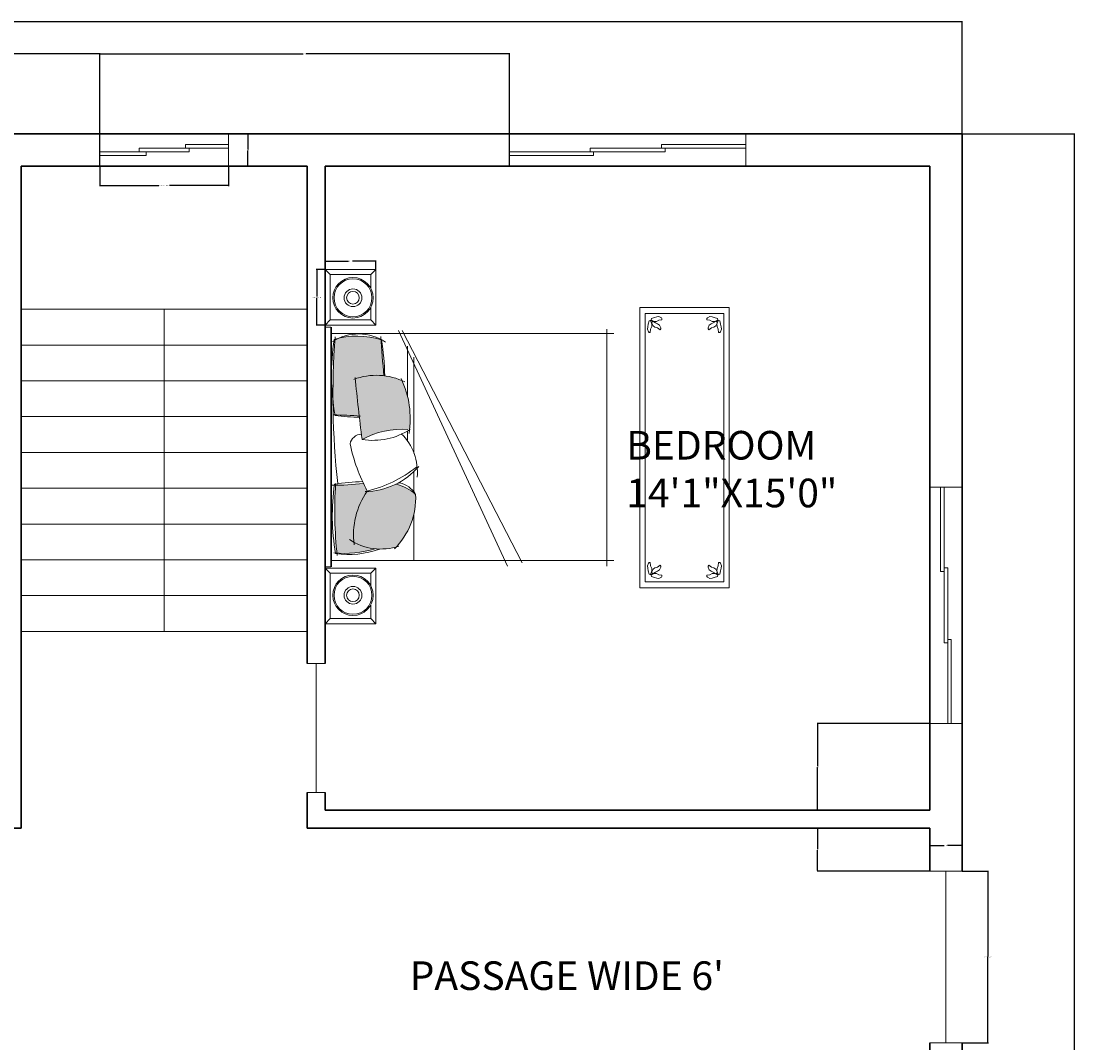
# Model space of a CAD drawing. Units: inches. Extents: x 1569 to 2779, y 1228 to 1844.
# Tile 4 of 6: x 1878 to 2173, y 1559 to 1844. Entities that reach past the tile are written whole.
import ezdxf

# ---------------------------------------------------------------- set-up
doc = ezdxf.new("R2010")
doc.units = ezdxf.units.IN
for name, color, linetype, lineweight in [('0.10', 252, 'Continuous', 9), ('0.15', 34, 'Continuous', 15), ('A-ANNO-DIMS', 2, 'Continuous', 18), ('A-AREA-IDEN', 7, 'Continuous', 18), ('A-DOOR', 3, 'Continuous', 20), ('A-FLOR-STRS', 4, 'Continuous', 18), ('A-FURN', 8, 'Continuous', 13), ('A-FURN-PATT', 116, 'Continuous', 9), ('A-GLAZ', 5, 'Continuous', 18), ('A-WALL', 7, 'Continuous', 35)]:
    doc.layers.add(name, color=color, linetype=linetype, lineweight=lineweight)
doc.styles.get("Standard").update_dxf_attribs({"font": 'arial.ttf'})
doc.dimstyles.get("Standard").update_dxf_attribs({"dimtxt": 0.18, "dimasz": 0.18, "dimexe": 0.18, "dimexo": 0.0625, "dimgap": 0.09, "dimtad": 0, "dimtih": 1, "dimtoh": 1, "dimdec": 4, "dimzin": 0, "dimdsep": 46, "dimtxsty": 'Standard', "dimcen": 0.09, "dimadec": 0, "dimazin": 0, "dimtfac": 1, "dimtdec": 4, "dimtofl": 0, "dimtmove": 0, "dimatfit": 3, "dimfxl": 1, "dimtolj": 1, "dimtzin": 0, "dimarcsym": 0})

# ---------------------------------------------------------------- blocks, each defined once
blk = doc.blocks.new('camita')
at = {"layer": '0.10'}
for p, q in [((-0.85, -0.045), (0.85, -0.045)), ((-0.805, -0.045), (-0.805, -2.0485)), ((0.805, -0.045), (0.805, -2.0485)), ((-0.8271, -0.521), (0.8464, -1.2932)), ((-0.8271, -0.5476), (0.8236, -1.3992)), ((-0.7161, -0.585), (-0.3554, -0.585)), ((-0.1136, -0.585), (-0.0485, -0.585)), ((-0.638, -0.63), (0.0434, -0.63)), ((0.1749, -0.63), (0.3179, -0.63)), ((0.4739, -0.63), (0.805, -0.63)), ((-0.8354, -2), (0.8464, -2))]:
    blk.add_line(p, q, dxfattribs=at)
blk.add_lwpolyline([(-0.85, -0.0405), (0.85, -0.0405), (0.85, 0), (-0.85, 0)], close=True, dxfattribs=at)
for centre, radius, start, end in [((-0.4574, -0.2364), 0.3443, 147.50996, 213.83359), ((-0.1997, -0.2266), 0.5864, 163.92635, 197.14087), ((-0.3639, -5.8457), 5.7909, 83.80731, 94.12107), ((-0.5104, -1.7232), 1.6781, 80.12554, 98.66187), ((2.3534, -0.0532), 2.5803, 180.10628, 184.38541), ((-1.5443, -0.2452), 1.3333, 359.93941, 7.55329), ((1.5815, -0.2893), 1.3353, 170.38021, 178.99138), ((-1.4396, -0.0609), 1.7117, 352.92911, 0.39592), ((0.4524, -3.0675), 2.9996, 83.90257, 93.67595), ((0.4863, -1.6286), 1.5781, 80.16015, 98.05996), ((0.0294, -0.1377), 0.7262, 342.58415, 6.00484), ((0.1326, -0.1696), 0.6307, 339.92303, 8.74334), ((-0.0543, -0.3633), 0.4542, 159.30257, 206.50263), ((-1.3301, -9.6748), 9.4985, 82.27078, 84.93989), ((-0.007, -0.258), 0.0828, 100.01798, 179.73597), ((-0.2931, -1.4378), 1.2903, 61.97485, 77.84351), ((0.6265, -0.7518), 0.5508, 82.96906, 124.67388), ((0.3203, -0.3944), 0.4043, 341.45245, 33.45121), ((0.4585, -0.5454), 0.5842, 151.04555, 184.14969), ((-0.5341, -0.3393), 0.4875, 327.26442, 9.0473), ((-0.1986, -0.2742), 0.5159, 310.73945, 359.05759), ((-0.5673, -0.0868), 0.9057, 321.69527, 346.46261), ((-1.8672, -14.986), 14.6323, 84.65974, 85.75157), ((-0.4598, 1.4861), 1.9092, 260.95299, 268.65169), ((0.5707, -0.4317), 0.3145, 192.93877, 221.96363), ((0.3612, -0.133), 0.5096, 267.25889, 315.29965), ((-0.2002, 0.064), 0.6673, 244.78094, 279.06058), ((0.179, -0.272), 0.3828, 224.52836, 275.22287), ((0.4384, -0.4834), 0.1898, 193.68485, 236.70352)]:
    blk.add_arc(centre, radius, start, end, dxfattribs=at)
blk = doc.blocks.new('VELADOR')
at = {"layer": '0.15'}
for p, q in [((-0.2475, 0), (-0.2025, -0.045)), ((0.2475, 0), (0.2025, -0.045)), ((-0.2025, -0.405), (-0.2475, -0.45)), ((0.2475, -0.45), (0.2025, -0.405))]:
    blk.add_line(p, q, dxfattribs=at)
blk.add_lwpolyline([(-0.2475, 0), (-0.2475, -0.45), (0.2475, -0.45), (0.2475, 0)], close=True, dxfattribs=at)
blk.add_lwpolyline([(0.0921, -0.405), (0.2025, -0.405), (0.2025, -0.045), (-0.2025, -0.045), (-0.2025, -0.405), (-0.0818, -0.405)], dxfattribs=at)
for radius in [0.18, 0.1688, 0.0788, 0.0563]:
    blk.add_circle((0.0052, -0.2474), radius, dxfattribs=at)
blk = doc.blocks.new('carpet-7')
at = {"color": 0, "linetype": 'ByBlock'}
for p, q in [((-1.0224, 0), (0, 0)), ((0, 0), (0, -0.54)), ((-1.694, -0.54), (-1.694, 0)), ((-1.694, 0), (-1.0224, 0)), ((-1.658, -0.5076), (-1.658, -0.0324)), ((-1.658, -0.0324), (-0.036, -0.0324)), ((-1.6112, -0.0562), (-1.6124, -0.0637)), ((-1.5896, -0.0518), (-1.6112, -0.0562)), ((-1.5752, -0.0486), (-1.5896, -0.0518)), ((-1.5608, -0.0464), (-1.5752, -0.0486)), ((-1.544, -0.0529), (-1.5608, -0.0464)), ((-1.5404, -0.0562), (-1.544, -0.0529)), ((-1.5404, -0.0637), (-1.5404, -0.0562)), ((-0.1512, -0.0562), (-0.1476, -0.0529)), ((-0.1512, -0.0637), (-0.1512, -0.0562)), ((-0.1476, -0.0529), (-0.1308, -0.0464)), ((-0.1308, -0.0464), (-0.1164, -0.0486)), ((-0.1164, -0.0486), (-0.102, -0.0518)), ((-0.102, -0.0518), (-0.0804, -0.0562)), ((-0.0804, -0.0562), (-0.0792, -0.0637)), ((-0.036, -0.0324), (-0.036, -0.5076)), ((-1.6364, -0.1156), (-1.634, -0.1026)), ((-1.6292, -0.1307), (-1.6364, -0.1156)), ((-1.634, -0.1026), (-1.6304, -0.0896)), ((-1.6304, -0.0896), (-1.6256, -0.0702)), ((-1.6256, -0.0702), (-1.6172, -0.0691)), ((-1.6172, -0.0691), (-1.6124, -0.0724)), ((-1.6148, -0.1156), (-1.6172, -0.1339)), ((-1.6076, -0.1015), (-1.6148, -0.1156)), ((-1.6124, -0.0637), (-1.6088, -0.068)), ((-1.6124, -0.0724), (-1.6064, -0.0886)), ((-1.6088, -0.068), (-1.5908, -0.0734)), ((-1.6088, -0.0788), (-1.6028, -0.0724)), ((-1.5992, -0.0961), (-1.6088, -0.0788)), ((-1.6064, -0.0886), (-1.6076, -0.1015)), ((-1.6028, -0.0724), (-1.5968, -0.0724)), ((-1.5932, -0.108), (-1.5992, -0.0961)), ((-1.5968, -0.0724), (-1.5812, -0.081)), ((-1.5848, -0.1199), (-1.5932, -0.108)), ((-1.5908, -0.0734), (-1.5764, -0.0724)), ((-1.5692, -0.1274), (-1.5848, -0.1199)), ((-1.5812, -0.081), (-1.5728, -0.0918)), ((-1.5764, -0.0724), (-1.5608, -0.0659)), ((-1.5728, -0.0918), (-1.568, -0.1069)), ((-1.568, -0.1069), (-1.5572, -0.1231)), ((-1.5572, -0.1231), (-1.5632, -0.1274)), ((-1.5608, -0.0659), (-1.5404, -0.0637)), ((-0.1308, -0.0659), (-0.1512, -0.0637)), ((-0.1236, -0.1069), (-0.1344, -0.1231)), ((-0.1344, -0.1231), (-0.1284, -0.1274)), ((-0.1152, -0.0724), (-0.1308, -0.0659)), ((-0.1188, -0.0918), (-0.1236, -0.1069)), ((-0.1224, -0.1274), (-0.1068, -0.1199)), ((-0.1104, -0.081), (-0.1188, -0.0918)), ((-0.1008, -0.0734), (-0.1152, -0.0724)), ((-0.0948, -0.0724), (-0.1104, -0.081)), ((-0.1068, -0.1199), (-0.0984, -0.108)), ((-0.0828, -0.068), (-0.1008, -0.0734)), ((-0.0984, -0.108), (-0.0924, -0.0961)), ((-0.0888, -0.0724), (-0.0948, -0.0724)), ((-0.0924, -0.0961), (-0.0828, -0.0788)), ((-0.0828, -0.0788), (-0.0888, -0.0724)), ((-0.0792, -0.0724), (-0.0852, -0.0886)), ((-0.0852, -0.0886), (-0.084, -0.1015)), ((-0.084, -0.1015), (-0.0768, -0.1156)), ((-0.0792, -0.0637), (-0.0828, -0.068)), ((-0.0744, -0.0691), (-0.0792, -0.0724)), ((-0.0768, -0.1156), (-0.0744, -0.1339)), ((-0.066, -0.0702), (-0.0744, -0.0691)), ((-0.0612, -0.0896), (-0.066, -0.0702)), ((-0.0624, -0.1307), (-0.0552, -0.1156)), ((-0.0576, -0.1026), (-0.0612, -0.0896)), ((-0.0552, -0.1156), (-0.0576, -0.1026)), ((-1.6256, -0.1339), (-1.6292, -0.1307)), ((-1.6172, -0.1339), (-1.6256, -0.1339)), ((-1.5632, -0.1274), (-1.5692, -0.1274)), ((-0.1284, -0.1274), (-0.1224, -0.1274)), ((-0.0744, -0.1339), (-0.066, -0.1339)), ((-0.066, -0.1339), (-0.0624, -0.1307)), ((-1.6292, -0.4093), (-1.6364, -0.4244)), ((-1.6364, -0.4244), (-1.634, -0.4374)), ((-1.634, -0.4374), (-1.6304, -0.4504)), ((-1.6256, -0.4061), (-1.6292, -0.4093)), ((-1.6172, -0.4061), (-1.6256, -0.4061)), ((-1.6148, -0.4244), (-1.6172, -0.4061)), ((-1.6076, -0.4385), (-1.6148, -0.4244)), ((-1.5992, -0.4439), (-1.6088, -0.4612)), ((-1.6064, -0.4514), (-1.6076, -0.4385)), ((-1.5932, -0.432), (-1.5992, -0.4439)), ((-1.5848, -0.4201), (-1.5932, -0.432)), ((-1.5692, -0.4126), (-1.5848, -0.4201)), ((-1.5728, -0.4482), (-1.568, -0.4331)), ((-1.5632, -0.4126), (-1.5692, -0.4126)), ((-1.568, -0.4331), (-1.5572, -0.4169)), ((-1.5572, -0.4169), (-1.5632, -0.4126)), ((-0.1344, -0.4169), (-0.1284, -0.4126)), ((-0.1236, -0.4331), (-0.1344, -0.4169)), ((-0.1284, -0.4126), (-0.1224, -0.4126)), ((-0.1188, -0.4482), (-0.1236, -0.4331)), ((-0.1224, -0.4126), (-0.1068, -0.4201)), ((-0.1068, -0.4201), (-0.0984, -0.432)), ((-0.0984, -0.432), (-0.0924, -0.4439)), ((-0.0924, -0.4439), (-0.0828, -0.4612)), ((-0.0852, -0.4514), (-0.084, -0.4385)), ((-0.084, -0.4385), (-0.0768, -0.4244)), ((-0.0768, -0.4244), (-0.0744, -0.4061)), ((-0.0744, -0.4061), (-0.066, -0.4061)), ((-0.066, -0.4061), (-0.0624, -0.4093)), ((-0.0624, -0.4093), (-0.0552, -0.4244)), ((-0.0576, -0.4374), (-0.0612, -0.4504)), ((-0.0552, -0.4244), (-0.0576, -0.4374)), ((-1.658, -0.5076), (-0.036, -0.5076)), ((-1.6304, -0.4504), (-1.6256, -0.4698)), ((-1.6256, -0.4698), (-1.6172, -0.4709)), ((-1.6172, -0.4709), (-1.6124, -0.4676)), ((-1.6124, -0.4676), (-1.6064, -0.4514)), ((-1.6124, -0.4763), (-1.6088, -0.472)), ((-1.6112, -0.4838), (-1.6124, -0.4763)), ((-1.5896, -0.4882), (-1.6112, -0.4838)), ((-1.6088, -0.4612), (-1.6028, -0.4676)), ((-1.6088, -0.472), (-1.5908, -0.4666)), ((-1.6028, -0.4676), (-1.5968, -0.4676)), ((-1.5968, -0.4676), (-1.5812, -0.459)), ((-1.5908, -0.4666), (-1.5764, -0.4676)), ((-1.5752, -0.4914), (-1.5896, -0.4882)), ((-1.5812, -0.459), (-1.5728, -0.4482)), ((-1.5764, -0.4676), (-1.5608, -0.4741)), ((-1.5608, -0.4936), (-1.5752, -0.4914)), ((-1.5608, -0.4741), (-1.5404, -0.4763)), ((-1.544, -0.4871), (-1.5608, -0.4936)), ((-1.5404, -0.4838), (-1.544, -0.4871)), ((-1.5404, -0.4763), (-1.5404, -0.4838)), ((-0.1308, -0.4741), (-0.1512, -0.4763)), ((-0.1512, -0.4763), (-0.1512, -0.4838)), ((-0.1512, -0.4838), (-0.1476, -0.4871)), ((-0.1476, -0.4871), (-0.1308, -0.4936)), ((-0.1152, -0.4676), (-0.1308, -0.4741)), ((-0.1308, -0.4936), (-0.1164, -0.4914)), ((-0.1104, -0.459), (-0.1188, -0.4482)), ((-0.1164, -0.4914), (-0.102, -0.4882)), ((-0.1008, -0.4666), (-0.1152, -0.4676)), ((-0.0948, -0.4676), (-0.1104, -0.459)), ((-0.102, -0.4882), (-0.0804, -0.4838)), ((-0.0828, -0.472), (-0.1008, -0.4666)), ((-0.0888, -0.4676), (-0.0948, -0.4676)), ((-0.0828, -0.4612), (-0.0888, -0.4676)), ((-0.0792, -0.4676), (-0.0852, -0.4514)), ((-0.0792, -0.4763), (-0.0828, -0.472)), ((-0.0804, -0.4838), (-0.0792, -0.4763)), ((-0.0744, -0.4709), (-0.0792, -0.4676)), ((-0.066, -0.4698), (-0.0744, -0.4709)), ((-0.0612, -0.4504), (-0.066, -0.4698)), ((0, -0.54), (-1.694, -0.54))]:
    blk.add_line(p, q, dxfattribs=at)
blk = doc.blocks.new('WIN-66IN')
for p, q in [((0, 0), (0, 9)), ((66, 0), (66, 9)), ((42.5, 6), (66, 6)), ((42.5, 5), (42.5, 6)), ((0, 4), (43.5, 4)), ((0, 3), (23.5, 3)), ((22.5, 5), (66, 5)), ((22.5, 4), (22.5, 5)), ((23.5, 3), (23.5, 4)), ((43.5, 4), (43.5, 5))]:
    blk.add_line(p, q)
blk = doc.blocks.new('WIN-36IN-A')
for p, q in [((0, 9), (0, 0)), ((36, 9), (36, 0)), ((24, 6), (24, 5)), ((36, 6), (24, 6)), ((25, 4), (0, 4)), ((13, 3), (0, 3)), ((36, 5), (11, 5)), ((11, 5), (11, 4)), ((13, 4), (13, 3)), ((25, 5), (25, 4))]:
    blk.add_line(p, q)
blk = doc.blocks.new('DOOR-48IN')
for p, q in [((0, 0), (0, 9)), ((48, 0), (48, 9)), ((48, 4.5), (0, 4.5))]:
    blk.add_line(p, q)
blk = doc.blocks.new('DOOR-36IN')
for p, q in [((0, 5), (0, 0)), ((36, 5), (36, 0)), ((36, 2.5), (0, 2.5))]:
    blk.add_line(p, q)
blk = doc.blocks.new('STAIR-RETURN-FLIGHT')
for p, q in [((80, 90), (0, 90)), ((40, 90), (40, 0)), ((80, 80), (0, 80)), ((80, 70), (0, 70)), ((80, 60), (0, 60)), ((80, 50), (0, 50)), ((80, 40), (0, 40)), ((80, 30), (0, 30)), ((80, 20), (0, 20)), ((80, 10), (0, 10)), ((80, 0), (0, 0))]:
    blk.add_line(p, q)
blk = doc.blocks.new('*D17')
at = {"layer": 'A-ANNO-DIMS', "color": 0, "lineweight": -2, "transparency": 16777216}
for p, q in [((2141.09, 1606.88), (2148.41, 1606.88)), ((2148.23, 1606.7), (2148.23, 1583.06)), ((2148.23, 1559.06), (2148.23, 1582.7)), ((2141.09, 1558.88), (2148.41, 1558.88))]:
    blk.add_line(p, q, dxfattribs=at)
at = {"layer": 'A-ANNO-DIMS', "color": 0, "transparency": 16777216}
for points in [[(2148.2, 1606.7), (2148.26, 1606.7), (2148.23, 1606.88)], [(2148.2, 1559.06), (2148.26, 1559.06), (2148.23, 1558.88)]]:
    blk.add_solid(points, dxfattribs=at)
at = {"layer": 'Defpoints', "color": 0, "transparency": 16777216}
for p in [(2141.03, 1606.88), (2148.23, 1606.88), (2141.03, 1558.88)]:
    blk.add_point(p, dxfattribs=at)
at = {"layer": 'A-ANNO-DIMS', "color": 0, "transparency": 16777216, "insert": (2148.23, 1582.88), "char_height": 0.18, "attachment_point": 5}
blk.add_mtext('\\A1;ENTRY DOOR 48 TYP.', dxfattribs=at)
blk = doc.blocks.new('*D18')
at = {"layer": 'A-ANNO-DIMS', "color": 0, "lineweight": -2, "transparency": 16777216}
for p, q in [((2132.03, 1606.94), (2132.03, 1614.26)), ((2141.03, 1606.94), (2141.03, 1614.26)), ((2132.21, 1614.08), (2136.07, 1614.08)), ((2140.85, 1614.08), (2136.99, 1614.08))]:
    blk.add_line(p, q, dxfattribs=at)
at = {"layer": 'A-ANNO-DIMS', "color": 0, "transparency": 16777216}
for points in [[(2132.21, 1614.11), (2132.21, 1614.05), (2132.03, 1614.08)], [(2140.85, 1614.11), (2140.85, 1614.05), (2141.03, 1614.08)]]:
    blk.add_solid(points, dxfattribs=at)
at = {"layer": 'Defpoints', "color": 0, "transparency": 16777216}
for p in [(2132.03, 1614.08), (2132.03, 1606.88), (2141.03, 1606.88)]:
    blk.add_point(p, dxfattribs=at)
at = {"layer": 'A-ANNO-DIMS', "color": 0, "transparency": 16777216, "insert": (2136.53, 1614.08), "char_height": 0.18, "attachment_point": 5}
blk.add_mtext('\\A1;9 TYP.', dxfattribs=at)
blk = doc.blocks.new('*D25')
at = {"layer": 'A-ANNO-DIMS', "color": 0, "lineweight": -2, "transparency": 16777216}
for p, q in [((1900.03, 1803.82), (1900.03, 1798.3)), ((1936.03, 1803.82), (1936.03, 1798.3)), ((1900.21, 1798.48), (1916.51, 1798.48)), ((1935.85, 1798.48), (1919.55, 1798.48))]:
    blk.add_line(p, q, dxfattribs=at)
at = {"layer": 'A-ANNO-DIMS', "color": 0, "transparency": 16777216}
for points in [[(1900.21, 1798.51), (1900.21, 1798.45), (1900.03, 1798.48)], [(1935.85, 1798.51), (1935.85, 1798.45), (1936.03, 1798.48)]]:
    blk.add_solid(points, dxfattribs=at)
at = {"layer": 'Defpoints', "color": 0, "transparency": 16777216}
for p in [(1900.03, 1803.88), (1936.03, 1803.88), (1936.03, 1798.48)]:
    blk.add_point(p, dxfattribs=at)
at = {"layer": 'A-ANNO-DIMS', "color": 0, "transparency": 16777216, "insert": (1918.03, 1798.48), "char_height": 0.18, "attachment_point": 5}
blk.add_mtext('\\A1;STAIR WINDOW 36 TYP.', dxfattribs=at)
blk = doc.blocks.new('*D26')
at = {"layer": 'A-ANNO-DIMS', "color": 0, "lineweight": -2, "transparency": 16777216}
for p, q in [((1936.09, 1812.88), (1941.61, 1812.88)), ((1941.43, 1812.7), (1941.43, 1808.56)), ((1941.43, 1804.06), (1941.43, 1808.2)), ((1936.09, 1803.88), (1941.61, 1803.88))]:
    blk.add_line(p, q, dxfattribs=at)
at = {"layer": 'A-ANNO-DIMS', "color": 0, "transparency": 16777216}
for points in [[(1941.4, 1812.7), (1941.46, 1812.7), (1941.43, 1812.88)], [(1941.4, 1804.06), (1941.46, 1804.06), (1941.43, 1803.88)]]:
    blk.add_solid(points, dxfattribs=at)
at = {"layer": 'Defpoints', "color": 0, "transparency": 16777216}
for p in [(1936.03, 1812.88), (1941.43, 1812.88), (1936.03, 1803.88)]:
    blk.add_point(p, dxfattribs=at)
at = {"layer": 'A-ANNO-DIMS', "color": 0, "transparency": 16777216, "insert": (1941.43, 1808.38), "char_height": 0.18, "attachment_point": 5}
blk.add_mtext('\\A1;9 TYP.', dxfattribs=at)
blk = doc.blocks.new('*D33')
at = {"layer": 'A-ANNO-DIMS', "color": 0, "lineweight": -2, "transparency": 16777216}
for p, q in [((1962.97, 1775.02), (1960.52, 1775.02)), ((1960.7, 1774.84), (1960.7, 1767.43)), ((1960.7, 1759.65), (1960.7, 1767.07)), ((1962.97, 1759.47), (1960.52, 1759.47))]:
    blk.add_line(p, q, dxfattribs=at)
at = {"layer": 'A-ANNO-DIMS', "color": 0, "transparency": 16777216}
for points in [[(1960.67, 1774.84), (1960.73, 1774.84), (1960.7, 1775.02)], [(1960.67, 1759.65), (1960.73, 1759.65), (1960.7, 1759.47)]]:
    blk.add_solid(points, dxfattribs=at)
at = {"layer": 'Defpoints', "color": 0, "transparency": 16777216}
for p in [(1963.03, 1775.02), (1960.7, 1759.47), (1963.03, 1759.47)]:
    blk.add_point(p, dxfattribs=at)
at = {"layer": 'A-ANNO-DIMS', "color": 0, "transparency": 16777216, "insert": (1960.7, 1767.25), "char_height": 0.18, "attachment_point": 5}
blk.add_mtext('\\A1;NIGHTSTAND 16 TYP.', dxfattribs=at)
blk = doc.blocks.new('*D34')
at = {"layer": 'A-ANNO-DIMS', "color": 0, "lineweight": -2, "transparency": 16777216}
for p, q in [((1963.03, 1775.09), (1963.03, 1777.54)), ((1963.21, 1777.36), (1969.58, 1777.36)), ((1976.99, 1777.36), (1970.62, 1777.36)), ((1977.17, 1775.09), (1977.17, 1777.54))]:
    blk.add_line(p, q, dxfattribs=at)
at = {"layer": 'A-ANNO-DIMS', "color": 0, "transparency": 16777216}
for points in [[(1963.21, 1777.39), (1963.21, 1777.33), (1963.03, 1777.36)], [(1976.99, 1777.39), (1976.99, 1777.33), (1977.17, 1777.36)]]:
    blk.add_solid(points, dxfattribs=at)
at = {"layer": 'Defpoints', "color": 0, "transparency": 16777216}
for p in [(1963.03, 1777.36), (1963.03, 1775.02), (1977.17, 1775.02)]:
    blk.add_point(p, dxfattribs=at)
at = {"layer": 'A-ANNO-DIMS', "color": 0, "transparency": 16777216, "insert": (1970.1, 1777.36), "char_height": 0.18, "attachment_point": 5}
blk.add_mtext('\\A1;14 TYP.', dxfattribs=at)
blk = doc.blocks.new('*D47')
at = {"layer": 'A-ANNO-DIMS', "color": 0, "lineweight": -2, "transparency": 16777216}
for p, q in [((1601.03, 1812.94), (1601.03, 1844.41)), ((1601.21, 1844.23), (1870.74, 1844.23)), ((2140.85, 1844.23), (1871.32, 1844.23)), ((2141.03, 1812.94), (2141.03, 1844.41))]:
    blk.add_line(p, q, dxfattribs=at)
at = {"layer": 'A-ANNO-DIMS', "color": 0, "transparency": 16777216}
for points in [[(1601.21, 1844.26), (1601.21, 1844.2), (1601.03, 1844.23)], [(2140.85, 1844.26), (2140.85, 1844.2), (2141.03, 1844.23)]]:
    blk.add_solid(points, dxfattribs=at)
at = {"layer": 'Defpoints', "color": 0, "transparency": 16777216}
for p in [(2141.03, 1844.23), (1601.03, 1812.88), (2141.03, 1812.88)]:
    blk.add_point(p, dxfattribs=at)
at = {"layer": 'A-ANNO-DIMS', "color": 0, "transparency": 16777216, "insert": (1871.03, 1844.23), "char_height": 0.18, "attachment_point": 5}
blk.add_mtext('\\A1;540', dxfattribs=at)
blk = doc.blocks.new('*D48')
at = {"layer": 'A-ANNO-DIMS', "color": 0, "lineweight": -2, "transparency": 16777216}
for p, q in [((2141.09, 1812.88), (2172.56, 1812.88)), ((2172.38, 1812.7), (2172.38, 1543.06)), ((2172.38, 1273.06), (2172.38, 1542.7)), ((2141.09, 1272.88), (2172.56, 1272.88))]:
    blk.add_line(p, q, dxfattribs=at)
at = {"layer": 'A-ANNO-DIMS', "color": 0, "transparency": 16777216}
for points in [[(2172.35, 1812.7), (2172.41, 1812.7), (2172.38, 1812.88)], [(2172.35, 1273.06), (2172.41, 1273.06), (2172.38, 1272.88)]]:
    blk.add_solid(points, dxfattribs=at)
at = {"layer": 'Defpoints', "color": 0, "transparency": 16777216}
for p in [(2141.03, 1812.88), (2172.38, 1812.88), (2141.03, 1272.88)]:
    blk.add_point(p, dxfattribs=at)
at = {"layer": 'A-ANNO-DIMS', "color": 0, "transparency": 16777216, "insert": (2172.38, 1542.88), "char_height": 0.18, "attachment_point": 5}
blk.add_mtext('\\A1;540', dxfattribs=at)
blk = doc.blocks.new('*D55')
at = {"layer": 'A-ANNO-DIMS', "color": 0, "lineweight": -2, "transparency": 16777216}
for p, q in [((1828.03, 1803.94), (1828.03, 1835.41)), ((1828.21, 1835.23), (1863.81, 1835.23)), ((1899.85, 1835.23), (1864.25, 1835.23)), ((1900.03, 1803.94), (1900.03, 1835.41))]:
    blk.add_line(p, q, dxfattribs=at)
at = {"layer": 'A-ANNO-DIMS', "color": 0, "transparency": 16777216}
for points in [[(1828.21, 1835.26), (1828.21, 1835.2), (1828.03, 1835.23)], [(1899.85, 1835.26), (1899.85, 1835.2), (1900.03, 1835.23)]]:
    blk.add_solid(points, dxfattribs=at)
at = {"layer": 'Defpoints', "color": 0, "transparency": 16777216}
for p in [(1900.03, 1835.23), (1828.03, 1803.88), (1900.03, 1803.88)]:
    blk.add_point(p, dxfattribs=at)
at = {"layer": 'A-ANNO-DIMS', "color": 0, "transparency": 16777216, "insert": (1864.03, 1835.23), "char_height": 0.18, "attachment_point": 5}
blk.add_mtext('\\A1;72', dxfattribs=at)
blk = doc.blocks.new('*D56')
at = {"layer": 'A-ANNO-DIMS', "color": 0, "lineweight": -2, "transparency": 16777216}
for p, q in [((1900.03, 1803.94), (1900.03, 1835.41)), ((1900.21, 1835.23), (1956.85, 1835.23)), ((2014.39, 1835.23), (1957.76, 1835.23)), ((2014.57, 1803.94), (2014.57, 1835.41))]:
    blk.add_line(p, q, dxfattribs=at)
at = {"layer": 'A-ANNO-DIMS', "color": 0, "transparency": 16777216}
for points in [[(1900.21, 1835.26), (1900.21, 1835.2), (1900.03, 1835.23)], [(2014.39, 1835.26), (2014.39, 1835.2), (2014.57, 1835.23)]]:
    blk.add_solid(points, dxfattribs=at)
at = {"layer": 'Defpoints', "color": 0, "transparency": 16777216}
for p in [(2014.57, 1835.23), (1900.03, 1803.88), (2014.57, 1803.88)]:
    blk.add_point(p, dxfattribs=at)
at = {"layer": 'A-ANNO-DIMS', "color": 0, "transparency": 16777216, "insert": (1957.3, 1835.23), "char_height": 0.18, "attachment_point": 5}
blk.add_mtext('\\A1;114.54', dxfattribs=at)
blk = doc.blocks.new('*D66')
at = {"layer": 'A-ANNO-DIMS', "color": 0, "lineweight": -2, "transparency": 16777216}
for p, q in [((2131.97, 1618.88), (2100.5, 1618.88)), ((2100.68, 1618.7), (2100.68, 1613.06)), ((2100.68, 1607.06), (2100.68, 1612.7)), ((2131.97, 1606.88), (2100.5, 1606.88))]:
    blk.add_line(p, q, dxfattribs=at)
at = {"layer": 'A-ANNO-DIMS', "color": 0, "transparency": 16777216}
for points in [[(2100.65, 1618.7), (2100.71, 1618.7), (2100.68, 1618.88)], [(2100.65, 1607.06), (2100.71, 1607.06), (2100.68, 1606.88)]]:
    blk.add_solid(points, dxfattribs=at)
at = {"layer": 'Defpoints', "color": 0, "transparency": 16777216}
for p in [(2100.68, 1618.88), (2132.03, 1618.88), (2132.03, 1606.88)]:
    blk.add_point(p, dxfattribs=at)
at = {"layer": 'A-ANNO-DIMS', "color": 0, "transparency": 16777216, "insert": (2100.68, 1612.88), "char_height": 0.18, "attachment_point": 5}
blk.add_mtext('\\A1;12', dxfattribs=at)
blk = doc.blocks.new('*D67')
at = {"layer": 'A-ANNO-DIMS', "color": 0, "lineweight": -2, "transparency": 16777216}
for p, q in [((2131.97, 1648.14), (2100.5, 1648.14)), ((2100.68, 1647.96), (2100.68, 1636.19)), ((2100.68, 1624.06), (2100.68, 1635.83)), ((2131.97, 1623.88), (2100.5, 1623.88))]:
    blk.add_line(p, q, dxfattribs=at)
at = {"layer": 'A-ANNO-DIMS', "color": 0, "transparency": 16777216}
for points in [[(2100.65, 1647.96), (2100.71, 1647.96), (2100.68, 1648.14)], [(2100.65, 1624.06), (2100.71, 1624.06), (2100.68, 1623.88)]]:
    blk.add_solid(points, dxfattribs=at)
at = {"layer": 'Defpoints', "color": 0, "transparency": 16777216}
for p in [(2100.68, 1648.14), (2132.03, 1648.14), (2132.03, 1623.88)]:
    blk.add_point(p, dxfattribs=at)
at = {"layer": 'A-ANNO-DIMS', "color": 0, "transparency": 16777216, "insert": (2100.68, 1636.01), "char_height": 0.18, "attachment_point": 5}
blk.add_mtext('\\A1;24.264', dxfattribs=at)

msp = doc.modelspace()

# ---------------------------------------------------------------- hatches: boundary and pattern name
at = {"layer": 'A-FURN-PATT'}
h = msp.add_hatch(color=256, dxfattribs=at)
h.dxf.hatch_style = 1
h.paths.add_polyline_path([(1978.6074, 1755.3888, 0.1310475), (1966.7154, 1755.7666, 0.02065708), (1965.7165, 1755.2602, 0.01851025), (1965.1921, 1738.3915, 0.01544243), (1965.7571, 1734.3504, -0.01670092), (1972.5371, 1734.0816, -0.00696723), (1971.4634, 1744.4488, -0.11389129), (1979.46, 1745.3149, -0.00438694)])
h.paths.add_polyline_path([(1965.9189, 1714.7076, 0.04021238), (1966.3023, 1695.7444, 0.09479225), (1976.9792, 1696.9632, -0.09848778), (1971.0375, 1698.7753, -0.17586366), (1974.7988, 1713.0866, -0.01174183), (1973.7275, 1715.2184, -0.02905141)])
h = msp.add_hatch(color=256, dxfattribs=at)
h.dxf.hatch_style = 1
h.paths.add_polyline_path([(1984.5483, 1743.9727, 0.18953567), (1971.4697, 1744.4952, 0.01140771), (1973.3783, 1727.5384, -0.1503613), (1986.618, 1730.3169, 0.13377603)])
h.paths.add_polyline_path([(1971.0438, 1698.8217, 0.1949524), (1982.9358, 1697.541, 0.20255928), (1988.3187, 1712.2024, 0.12732633), (1982.8112, 1715.0635, -0.10404536), (1974.7085, 1712.9922, 0.17383481)])

# ---------------------------------------------------------------- linework, layer by layer
at = {"layer": 'A-WALL'}
for p, q in [((2141.032, 1812.8785), (1601.032, 1812.8785)), ((2141.032, 1606.8785), (2141.032, 1812.8785)), ((1878.032, 1803.8785), (1878.032, 1618.8785)), ((1958.032, 1803.8785), (1878.032, 1803.8785)), ((1958.032, 1664.8785), (1958.032, 1803.8785)), ((2132.032, 1803.8785), (1963.032, 1803.8785)), ((1963.032, 1664.8785), (1963.032, 1803.8785)), ((2132.032, 1623.8785), (2132.032, 1803.8785)), ((1958.032, 1618.8785), (1958.032, 1628.8785)), ((1963.032, 1623.8785), (1963.032, 1628.8785)), ((2132.032, 1623.8785), (1963.032, 1623.8785)), ((1878.032, 1618.8785), (1797.032, 1618.8785)), ((2132.032, 1618.8785), (1958.032, 1618.8785)), ((2132.032, 1606.8785), (2132.032, 1618.8785)), ((2132.032, 1546.8785), (2132.032, 1558.8785)), ((2141.032, 1272.8785), (2141.032, 1558.8785))]:
    msp.add_line(p, q, dxfattribs=at)

# ---------------------------------------------------------------- block references
at = {"layer": 'A-DOOR'}
for name, p, rotation in [('DOOR-36IN', (1958.032, 1664.8785), 270), ('DOOR-48IN', (2141.032, 1558.8785), 89.99999999999801)]:
    msp.add_blockref(name, p, dxfattribs=dict(at, rotation=rotation))
at = {"layer": 'A-FLOR-STRS'}
msp.add_blockref('STAIR-RETURN-FLIGHT', (1878.032, 1673.8785), dxfattribs=at)
at = {"layer": 'A-FURN'}
for name, p, xscale, yscale, zscale, rotation in [('VELADOR', (1963.032, 1767.2493), -31.41542173157097, 31.41542173157097, 31.41542173157097, 90), ('carpet-7', (2050.9482, 1764.3962), 46.2750735389499, 46.2750735389499, 46.2750735389499, 90), ('camita', (1963.032, 1725.418), -39.375, 39.375, 39.375, 90), ('VELADOR', (1963.032, 1683.7999), 31.41542173157097, 31.41542173157097, 31.41542173157097, 90.00000000000011)]:
    msp.add_blockref(name, p, dxfattribs=dict(at, xscale=xscale, yscale=yscale, zscale=zscale, rotation=rotation))
at = {"layer": 'A-GLAZ'}
for name, p in [('WIN-36IN-A', (1900.032, 1803.8785)), ('WIN-66IN', (2014.5712, 1803.8785))]:
    msp.add_blockref(name, p, dxfattribs=at)
at = {"layer": 'A-GLAZ', "rotation": 269.9999999999992}
msp.add_blockref('WIN-66IN', (2132.032, 1714.1428), dxfattribs=at)

# ---------------------------------------------------------------- texts
at = {"layer": 'A-AREA-IDEN', "char_height": 8, "attachment_point": 1}
for s, insert in [('BEDROOM\\P14\'1"X15\'0"', (2047.1869, 1729.8853)), (" PASSAGE WIDE 6'", (1984.2, 1581.6707))]:
    msp.add_mtext_dynamic_manual_height_columns(s, width=101.861325, gutter_width=12.5, heights=[0], dxfattribs=dict(at, insert=insert))

# ---------------------------------------------------------------- dimensions: what is measured, and where the dimension line sits
at = {"layer": 'A-ANNO-DIMS'}
for base, p1, p2, override, picture, middle in [((2141.032, 1844.2285), (1601.032, 1812.8785), (2141.032, 1812.8785), {"dimdec": 0, "dimlfac": 1, "dimrnd": 0, "dimzin": 0, "dimdsep": 46, "dimlunit": 2}, '*D47', (1871.032, 1844.2285)), ((1900.032, 1835.2285), (1828.032, 1803.8785), (1900.032, 1803.8785), {"dimdec": 0, "dimlfac": 1, "dimrnd": 0, "dimzin": 0, "dimdsep": 46, "dimlunit": 2}, '*D55', (1864.032, 1835.2285)), ((2014.5712, 1835.2285), (1900.032, 1803.8785), (2014.5712, 1803.8785), {"dimdec": 2, "dimlfac": 1, "dimrnd": 0, "dimzin": 0, "dimdsep": 46, "dimlunit": 2}, '*D56', (1957.3016, 1835.2285))]:
    dim = msp.add_linear_dim(base=base, p1=p1, p2=p2, dimstyle='Standard', override=override, dxfattribs=at)
    dim.commit()
    dim.dimension.update_dxf_attribs({"geometry": picture, "text_midpoint": middle})
for base, p1, p2, angle, text, picture, middle in [((1941.432, 1812.8785), (1936.032, 1803.8785), (1936.032, 1812.8785), 90, '<> TYP.', '*D26', (1941.432, 1808.3785)), ((1963.032, 1777.3572), (1977.169, 1775.0246), (1963.032, 1775.0246), 180, '<> TYP.', '*D34', (1970.1005, 1777.3572)), ((1960.6994, 1759.4739), (1963.032, 1775.0246), (1963.032, 1759.4739), 270, 'NIGHTSTAND <> TYP.', '*D33', (1960.6994, 1767.2493)), ((2132.032, 1614.0785), (2141.032, 1606.8785), (2132.032, 1606.8785), 180, '<> TYP.', '*D18', (2136.532, 1614.0785)), ((2148.232, 1606.8785), (2141.032, 1558.8785), (2141.032, 1606.8785), 90, 'ENTRY DOOR <> TYP.', '*D17', (2148.232, 1582.8785))]:
    dim = msp.add_linear_dim(base=base, p1=p1, p2=p2, angle=angle, text=text, dimstyle='Standard', override={"dimdec": 0, "dimlfac": 1, "dimrnd": 0, "dimzin": 0, "dimdsep": 46, "dimlunit": 2}, dxfattribs=at)
    dim.commit()
    dim.dimension.update_dxf_attribs({"geometry": picture, "text_midpoint": middle})
for base, p1, p2, override, picture, middle in [((2172.382, 1812.8785), (2141.032, 1272.8785), (2141.032, 1812.8785), {"dimdec": 0, "dimlfac": 1, "dimrnd": 0, "dimzin": 0, "dimdsep": 46, "dimlunit": 2}, '*D48', (2172.382, 1542.8785)), ((2100.682, 1648.1428), (2132.032, 1623.8785), (2132.032, 1648.1428), {"dimdec": 3, "dimlfac": 1, "dimrnd": 0, "dimzin": 0, "dimdsep": 46, "dimlunit": 2}, '*D67', (2100.682, 1636.0106)), ((2100.682, 1618.8785), (2132.032, 1606.8785), (2132.032, 1618.8785), {"dimdec": 0, "dimlfac": 1, "dimrnd": 0, "dimzin": 0, "dimdsep": 46, "dimlunit": 2}, '*D66', (2100.682, 1612.8785))]:
    dim = msp.add_linear_dim(base=base, p1=p1, p2=p2, angle=90, dimstyle='Standard', override=override, dxfattribs=at)
    dim.commit()
    dim.dimension.update_dxf_attribs({"geometry": picture, "text_midpoint": middle})
dim = msp.add_linear_dim(base=(1936.032, 1798.4785), p1=(1900.032, 1803.8785), p2=(1936.032, 1803.8785), text='STAIR WINDOW <> TYP.', dimstyle='Standard', override={"dimdec": 0, "dimlfac": 1, "dimrnd": 0, "dimzin": 0, "dimdsep": 46, "dimlunit": 2}, dxfattribs=at)
dim.commit()
dim.dimension.update_dxf_attribs({"geometry": '*D25', "text_midpoint": (1918.032, 1798.4785)})

doc.saveas('drawing.dxf')
